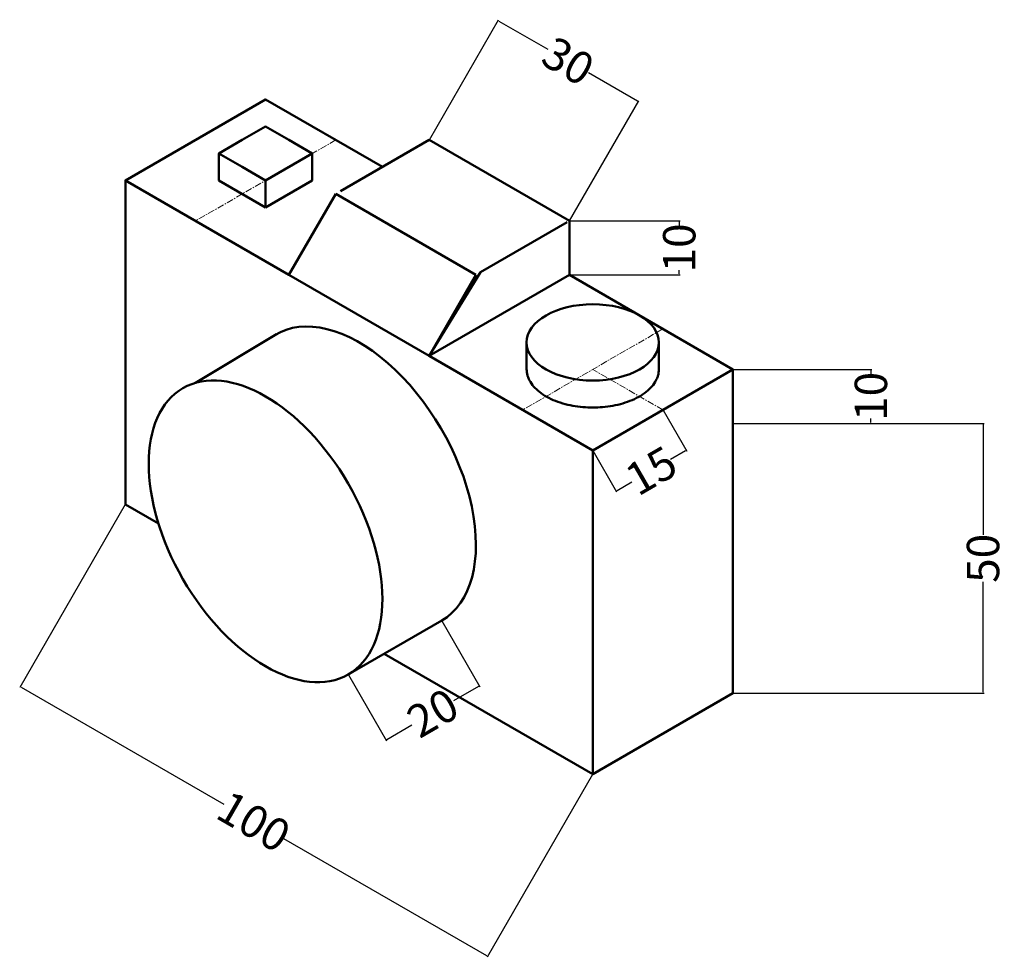
# Model space of a CAD drawing. Units: millimetres. Extents: x -20 to 162, y -21 to 153.
import ezdxf

# ---------------------------------------------------------------- set-up
doc = ezdxf.new("R2010")
doc.units = ezdxf.units.MM
doc.header["$MEASUREMENT"] = 0
doc.linetypes.add('CENTER', pattern=[2, 1.25, -0.25, 0.25, -0.25])
for name, color, linetype, lineweight in [('M-CNTR', 1, 'CENTER', 18), ('M-DIMS', 2, 'Continuous', 25), ('M-OUTL', 7, 'Continuous', 50)]:
    doc.layers.add(name, color=color, linetype=linetype, lineweight=lineweight)
doc.styles.get("Standard").update_dxf_attribs({"font": 'arial.ttf'})
doc.dimstyles.get("Standard").update_dxf_attribs({"dimtxt": 6, "dimasz": 0.18, "dimexe": 0.18, "dimexo": 0.0625, "dimgap": 0.09, "dimtad": 0, "dimtoh": 1, "dimdec": 0, "dimzin": 0, "dimdsep": 46, "dimtxsty": 'Standard', "dimcen": 0.09, "dimadec": 0, "dimazin": 0, "dimtfac": 1, "dimtdec": 0, "dimtofl": 0, "dimtmove": 0, "dimatfit": 3, "dimfxl": 1, "dimtolj": 1, "dimtzin": 0, "dimarcsym": 0})

# ---------------------------------------------------------------- blocks, each defined once
blk = doc.blocks.new('*D1')
at = {"layer": 'Defpoints', "color": 0, "transparency": 16777216}
for p in [(94.61, 137.38), (55.86, 130.25), (81.84, 115.25)]:
    blk.add_point(p, dxfattribs=at)
at = {"layer": 'M-DIMS', "color": 0, "lineweight": -2, "transparency": 16777216}
for p, q in [((55.89, 130.3), (68.72, 152.53)), ((68.79, 152.28), (77.83, 147.06)), ((94.46, 137.46), (85.41, 142.69)), ((81.87, 115.3), (94.7, 137.53))]:
    blk.add_line(p, q, dxfattribs=at)
at = {"layer": 'M-DIMS', "color": 0, "transparency": 16777216}
for points in [[(68.8, 152.31), (68.77, 152.26), (68.63, 152.37)], [(94.47, 137.49), (94.44, 137.44), (94.61, 137.38)]]:
    blk.add_solid(points, dxfattribs=at)
at = {"layer": 'M-DIMS', "color": 0, "transparency": 16777216, "insert": (81.62, 144.87), "char_height": 6, "attachment_point": 5, "rotation": 330}
blk.add_mtext('\\A1;30', dxfattribs=at)
blk = doc.blocks.new('*D2')
at = {"layer": 'Defpoints', "color": 0, "transparency": 16777216}
for p in [(112.15, 87.75), (112.15, 77.75), (137.7, 77.75)]:
    blk.add_point(p, dxfattribs=at)
at = {"layer": 'M-DIMS', "color": 0, "lineweight": -2, "transparency": 16777216}
for p, q in [((112.21, 87.75), (137.88, 87.75)), ((137.7, 87.57), (137.7, 86.84)), ((137.7, 77.93), (137.7, 78.66)), ((112.21, 77.75), (137.88, 77.75))]:
    blk.add_line(p, q, dxfattribs=at)
at = {"layer": 'M-DIMS', "color": 0, "transparency": 16777216}
for points in [[(137.67, 87.57), (137.73, 87.57), (137.7, 87.75)], [(137.67, 77.93), (137.73, 77.93), (137.7, 77.75)]]:
    blk.add_solid(points, dxfattribs=at)
at = {"layer": 'M-DIMS', "color": 0, "transparency": 16777216, "insert": (137.7, 82.75), "char_height": 6, "attachment_point": 5, "rotation": 90}
blk.add_mtext('\\A1;10', dxfattribs=at)
blk = doc.blocks.new('*D3')
at = {"layer": 'Defpoints', "color": 0, "transparency": 16777216}
for p in [(112.15, 77.75), (112.15, 27.75), (158.48, 27.75)]:
    blk.add_point(p, dxfattribs=at)
at = {"layer": 'M-DIMS', "color": 0, "lineweight": -2, "transparency": 16777216}
for p, q in [((112.21, 77.75), (158.66, 77.75)), ((158.48, 77.57), (158.48, 57.13)), ((158.48, 27.93), (158.48, 48.37)), ((112.21, 27.75), (158.66, 27.75))]:
    blk.add_line(p, q, dxfattribs=at)
at = {"layer": 'M-DIMS', "color": 0, "transparency": 16777216}
for points in [[(158.45, 77.57), (158.51, 77.57), (158.48, 77.75)], [(158.45, 27.93), (158.51, 27.93), (158.48, 27.75)]]:
    blk.add_solid(points, dxfattribs=at)
at = {"layer": 'M-DIMS', "color": 0, "transparency": 16777216, "insert": (158.48, 52.75), "char_height": 6, "attachment_point": 5, "rotation": 90}
blk.add_mtext('\\A1;50', dxfattribs=at)
blk = doc.blocks.new('*D4')
at = {"layer": 'Defpoints', "color": 0, "transparency": 16777216}
for p in [(99.16, 80.25), (86.17, 72.75), (90.5, 65.25)]:
    blk.add_point(p, dxfattribs=at)
at = {"layer": 'M-DIMS', "color": 0, "lineweight": -2, "transparency": 16777216}
for p, q in [((99.19, 80.2), (103.58, 72.59)), ((86.2, 72.7), (90.59, 65.09)), ((103.33, 72.66), (100.57, 71.06)), ((90.66, 65.34), (93.42, 66.94))]:
    blk.add_line(p, q, dxfattribs=at)
at = {"layer": 'M-DIMS', "color": 0, "transparency": 16777216}
for points in [[(103.32, 72.69), (103.35, 72.63), (103.49, 72.75)], [(90.64, 65.37), (90.67, 65.31), (90.5, 65.25)]]:
    blk.add_solid(points, dxfattribs=at)
at = {"layer": 'M-DIMS', "color": 0, "transparency": 16777216, "insert": (96.99, 69), "char_height": 6, "attachment_point": 5, "rotation": 30}
blk.add_mtext('\\A1;15', dxfattribs=at)
blk = doc.blocks.new('*D5')
at = {"layer": 'Defpoints', "color": 0, "transparency": 16777216}
for p in [(58.18, 41.23), (40.86, 31.23), (65.17, 29.12)]:
    blk.add_point(p, dxfattribs=at)
at = {"layer": 'M-DIMS', "color": 0, "lineweight": -2, "transparency": 16777216}
for p, q in [((58.21, 41.18), (65.26, 28.97)), ((40.89, 31.18), (47.94, 18.97)), ((65.01, 29.03), (60.34, 26.34)), ((48, 19.21), (52.67, 21.91))]:
    blk.add_line(p, q, dxfattribs=at)
at = {"layer": 'M-DIMS', "color": 0, "transparency": 16777216}
for points in [[(65, 29.06), (65.03, 29.01), (65.17, 29.12)], [(47.99, 19.24), (48.02, 19.19), (47.85, 19.12)]]:
    blk.add_solid(points, dxfattribs=at)
at = {"layer": 'M-DIMS', "color": 0, "transparency": 16777216, "insert": (56.51, 24.12), "char_height": 6, "attachment_point": 5, "rotation": 30}
blk.add_mtext('\\A1;20', dxfattribs=at)
blk = doc.blocks.new('*D6')
at = {"layer": 'Defpoints', "color": 0, "transparency": 16777216}
for p in [(81.84, 115.25), (81.84, 105.25), (102.19, 105.25)]:
    blk.add_point(p, dxfattribs=at)
at = {"layer": 'M-DIMS', "color": 0, "lineweight": -2, "transparency": 16777216}
for p, q in [((81.9, 115.25), (102.37, 115.25)), ((102.19, 115.07), (102.19, 114.34)), ((102.19, 105.43), (102.19, 106.16)), ((81.9, 105.25), (102.37, 105.25))]:
    blk.add_line(p, q, dxfattribs=at)
at = {"layer": 'M-DIMS', "color": 0, "transparency": 16777216}
for points in [[(102.16, 115.07), (102.22, 115.07), (102.19, 115.25)], [(102.16, 105.43), (102.22, 105.43), (102.19, 105.25)]]:
    blk.add_solid(points, dxfattribs=at)
at = {"layer": 'M-DIMS', "color": 0, "transparency": 16777216, "insert": (102.19, 110.25), "char_height": 6, "attachment_point": 5, "rotation": 90}
blk.add_mtext('\\A1;10', dxfattribs=at)
blk = doc.blocks.new('*D7')
at = {"layer": 'Defpoints', "color": 0, "transparency": 16777216}
for p in [(-0.43, 62.75), (86.17, 12.75), (66.68, -21)]:
    blk.add_point(p, dxfattribs=at)
at = {"layer": 'M-DIMS', "color": 0, "lineweight": -2, "transparency": 16777216}
for p, q in [((-0.46, 62.7), (-20.01, 28.84)), ((-19.76, 28.91), (17.82, 7.21)), ((86.14, 12.7), (66.59, -21.16)), ((66.53, -20.91), (28.95, 0.79))]:
    blk.add_line(p, q, dxfattribs=at)
at = {"layer": 'M-DIMS', "color": 0, "transparency": 16777216}
for points in [[(-19.75, 28.94), (-19.78, 28.88), (-19.92, 29)], [(66.54, -20.88), (66.51, -20.94), (66.68, -21)]]:
    blk.add_solid(points, dxfattribs=at)
at = {"layer": 'M-DIMS', "color": 0, "transparency": 16777216, "insert": (23.38, 4), "char_height": 6, "attachment_point": 5, "rotation": 330}
blk.add_mtext('\\A1;100', dxfattribs=at)

msp = doc.modelspace()

# ---------------------------------------------------------------- linework, layer by layer
at = {"layer": 'M-CNTR'}
for p, q in [((38.54, 130.25), (12.56, 115.25)), ((99.16, 95.25), (73.18, 80.25)), ((99.16, 80.25), (86.17, 87.75))]:
    msp.add_line(p, q, dxfattribs=at)
at = {"layer": 'M-OUTL'}
for p, q in [((16.89, 127.75), (16.89, 122.75)), ((34.21, 127.75), (34.21, 122.75)), ((29.88, 105.25), (-0.43, 122.75)), ((25.55, 117.75), (16.89, 122.75)), ((25.55, 117.75), (34.21, 122.75)), ((25.55, 117.75), (25.55, 122.75)), ((38.54, 120.25), (29.88, 105.25)), ((64.52, 105.25), (38.54, 120.25)), ((55.86, 90.25), (29.88, 105.25)), ((64.52, 105.25), (55.86, 90.25)), ((27.56, 94.27), (12.56, 85.25)), ((86.17, 72.75), (55.86, 90.25)), ((86.17, 72.75), (112.15, 87.75)), ((86.17, 12.75), (86.17, 72.75)), ((40.86, 31.23), (58.18, 41.23))]:
    msp.add_line(p, q, dxfattribs=at)
for points in [[(47.2, 125.25), (25.55, 137.75), (-0.43, 122.75), (-0.43, 62.75), (5.7, 59.21)], [(81.84, 105.25), (81.84, 115.25), (55.86, 130.25), (39.4, 120.75)], [(47.51, 35.07), (86.17, 12.75), (112.15, 27.75), (112.15, 77.75), (112.15, 87.75), (81.84, 105.25), (55.86, 90.25), (65.38, 105.75), (81.41, 115)]]:
    msp.add_lwpolyline(points, dxfattribs=at)
msp.add_lwpolyline([(25.55, 132.75), (21.22, 130.25), (16.89, 127.75), (21.22, 125.25), (25.55, 122.75), (34.21, 127.75), (29.88, 130.25)], close=True, dxfattribs=at)
for centre, major_axis in [((86.17, 92.75), (-12.25, 0)), ((25.55, 57.75), (15.31, -26.52))]:
    msp.add_ellipse(centre, major_axis=major_axis, ratio=0.57735, dxfattribs=at)
msp.add_ellipse((42.87, 67.75), major_axis=(15.31, -26.52), ratio=0.57735, start_param=6.283185, end_param=9.445082, dxfattribs=at)
msp.add_rational_spline([(73.92, 92.75), (73.92, 90.25), (73.92, 87.75), (73.92, 80.68), (86.17, 80.68), (98.42, 80.68), (98.42, 87.75), (98.42, 90.25), (98.42, 92.75)], [1, 1, 1, 0.707106781187, 1, 0.707106781187, 1, 1, 1], degree=2, knots=[0, 0, 0, 1, 1, 2.570796, 2.570796, 4.141593, 4.141593, 5.141593, 5.141593, 5.141593], dxfattribs=at)

# ---------------------------------------------------------------- dimensions: what is measured, and where the dimension line sits
at = {"layer": 'M-DIMS'}
for p1, p2, distance, picture, middle in [((55.86, 130.25), (81.84, 115.25), 25.55, '*D1', (81.62, 144.87)), ((81.84, 115.25), (81.84, 105.25), 20.35, '*D6', (102.19, 110.25)), ((112.15, 87.75), (112.15, 77.75), 25.55, '*D2', (137.7, 82.75)), ((99.16, 80.25), (86.17, 72.75), 8.66, '*D4', (96.99, 69)), ((112.15, 77.75), (112.15, 27.75), 46.33, '*D3', (158.48, 52.75)), ((-0.43, 62.75), (86.17, 12.75), -38.97, '*D7', (23.38, 4)), ((40.86, 31.23), (58.18, 41.23), -13.98, '*D5', (56.51, 24.12))]:
    dim = msp.add_aligned_dim(p1=p1, p2=p2, distance=distance, dimstyle='Standard', override={"dimclrd": 0, "dimclre": 0, "dimclrt": 0}, dxfattribs=at)
    dim.commit()
    dim.dimension.update_dxf_attribs({"geometry": picture, "text_midpoint": middle})

doc.saveas('drawing.dxf')
